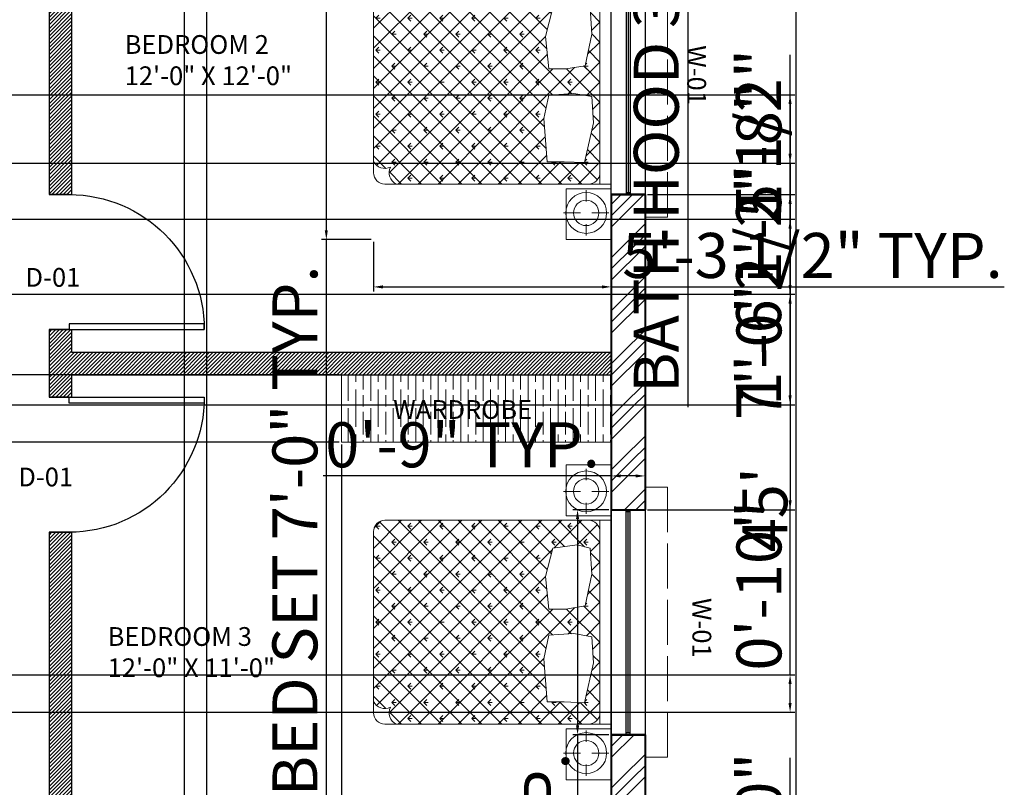
# Model space of a CAD drawing. Units: inches. Extents: x 2386 to 3029, y 792 to 1465.
# Tile 11 of 12: x 2724 to 2987, y 1044 to 1249. Entities that reach past the tile are written whole.
import ezdxf

# ---------------------------------------------------------------- set-up
doc = ezdxf.new("R2010")
doc.units = ezdxf.units.IN
doc.linetypes.add('ACAD_ISO02W100', pattern=[15, 12, -3])
for name, color, linetype, lineweight in [('A-AREA-IDEN', 4, 'Continuous', 25), ('A-DIMS', 1, 'Continuous', 18), ('A-DOOR', 2, 'Continuous', 25), ('A-FLOR-CASE', 6, 'Continuous', 18), ('A-FLOR-CASE-PATT', 9, 'Continuous', 13), ('A-FURN', 6, 'Continuous', 18), ('A-TEXT', 4, 'Continuous', 25), ('A-WALL-EXT', 7, 'Continuous', 40), ('A-WALL-INT', 9, 'Continuous', 30), ('A-WALL-PATT', 9, 'Continuous', 13), ('A-WINDOW', 4, 'Continuous', 25), ('A-WINDOW-OVHD', 4, 'ACAD_ISO02W100', 18)]:
    doc.layers.add(name, color=color, linetype=linetype, lineweight=lineweight)
doc.styles.get("Standard").update_dxf_attribs({"font": 'arial.ttf'})
doc.dimstyles.new('ISO-25', dxfattribs={"dimtxt": 12, "dimasz": 2.5, "dimexe": 1.25, "dimexo": 0.625, "dimtad": 1, "dimlunit": 4, "dimtxsty": 'Standard', "dimcen": 2.5, "dimadec": 0, "dimazin": 0, "dimtfac": 1, "dimtmove": 0, "dimatfit": 3, "dimfxl": 1, "dimarcsym": 0})

# ---------------------------------------------------------------- blocks, each defined once
blk = doc.blocks.new('*X5')
at = {"color": 0}
for p, q in [((0, 0), (0, 0)), ((-565.7, 0), (-565.7, 0)), ((-565.7, 0), (-565.7, 0)), ((-282.8, 0), (-282.8, 0)), ((-282.8, 0), (-282.8, 0)), ((282.8, 0), (282.8, 0)), ((565.7, 0), (565.7, 0)), ((-707.1, -141.4), (-733.6, -114.9)), ((-707.1, -141.4), (-707.1, -103.9)), ((-707.1, -141.4), (-680.6, -114.9)), ((-156.4, -126.5), (-167.9, -114.9)), ((-141.4, -141.4), (-142.5, -140.4)), ((-141.4, -141.4), (-141.4, -103.9)), ((-141.4, -141.4), (-114.9, -114.9)), ((119.7, -119.7), (114.9, -114.9)), ((699.4, -133.7), (680.6, -114.9)), ((707.1, -135.4), (707.1, -103.9)), ((710, -138.6), (733.6, -114.9)), ((-848.5, -282.8), (-875, -256.3)), ((-848.5, -282.8), (-848.5, -245.3)), ((-848.5, -282.8), (-822, -256.3)), ((0, -282.8), (-26.5, -256.3)), ((0, -282.8), (0, -245.3)), ((0, -282.8), (26.5, -256.3)), ((848.5, -282.8), (822, -256.3)), ((848.5, -282.8), (848.5, -245.3)), ((848.5, -282.8), (875, -256.3)), ((-707.1, -424.3), (-733.6, -397.7)), ((-707.1, -424.3), (-707.1, -386.8)), ((-707.1, -424.3), (-680.6, -397.7)), ((-115.7, -398.5), (-114.9, -397.7)), ((707.1, -424.3), (702.9, -420)), ((707.1, -424.3), (707.1, -386.8)), ((707.1, -424.3), (733.6, -397.7)), ((-848.5, -565.7), (-875, -539.2)), ((-848.5, -565.7), (-848.5, -528.2)), ((-848.5, -565.7), (-822, -539.2)), ((-565.7, -565.7), (-592.2, -539.2)), ((-565.7, -565.7), (-565.7, -528.2)), ((-565.7, -565.7), (-539.2, -539.2)), ((-282.8, -565.7), (-309.4, -539.2)), ((-282.8, -565.7), (-282.8, -528.2)), ((-282.8, -565.7), (-256.3, -539.2)), ((0, -565.7), (-26.5, -539.2)), ((0, -565.7), (0, -528.2)), ((0, -565.7), (26.5, -539.2)), ((282.8, -565.7), (256.3, -539.2)), ((282.8, -565.7), (282.8, -528.2)), ((282.8, -565.7), (309.4, -539.2)), ((565.7, -565.7), (539.2, -539.2)), ((565.7, -565.7), (565.7, -528.2)), ((565.7, -565.7), (592.2, -539.2)), ((848.5, -565.7), (822, -539.2)), ((848.5, -565.7), (848.5, -528.2)), ((848.5, -565.7), (875, -539.2)), ((-707.1, -707.1), (-733.6, -680.6)), ((-707.1, -707.1), (-707.1, -669.6)), ((-707.1, -707.1), (-680.6, -680.6)), ((-424.3, -707.1), (-450.8, -680.6)), ((-424.3, -707.1), (-424.3, -669.6)), ((-424.3, -707.1), (-397.7, -680.6)), ((-141.4, -707.1), (-167.9, -680.6)), ((-141.4, -707.1), (-141.4, -669.6)), ((-141.4, -707.1), (-114.9, -680.6)), ((141.4, -707.1), (114.9, -680.6)), ((141.4, -707.1), (141.4, -669.6)), ((141.4, -707.1), (167.9, -680.6)), ((424.3, -707.1), (397.7, -680.6)), ((424.3, -707.1), (424.3, -669.6)), ((424.3, -707.1), (450.8, -680.6)), ((707.1, -707.1), (680.6, -680.6)), ((707.1, -707.1), (707.1, -669.6)), ((707.1, -707.1), (733.6, -680.6)), ((-848.5, -848.5), (-875, -822)), ((-848.5, -848.5), (-848.5, -811)), ((-848.5, -848.5), (-822, -822)), ((-565.7, -848.5), (-592.2, -822)), ((-565.7, -848.5), (-565.7, -811)), ((-565.7, -848.5), (-539.2, -822)), ((-282.8, -848.5), (-309.4, -822)), ((-282.8, -848.5), (-282.8, -811)), ((-282.8, -848.5), (-256.3, -822)), ((0, -848.5), (-26.5, -822)), ((0, -848.5), (0, -811)), ((0, -848.5), (26.5, -822)), ((282.8, -848.5), (256.3, -822)), ((282.8, -848.5), (282.8, -811)), ((282.8, -848.5), (309.4, -822)), ((565.7, -848.5), (539.2, -822)), ((565.7, -848.5), (565.7, -811)), ((565.7, -848.5), (592.2, -822)), ((848.5, -848.5), (822, -822)), ((848.5, -848.5), (848.5, -811)), ((848.5, -848.5), (875, -822)), ((-707.1, -989.9), (-707.1, -952.4)), ((-424.3, -989.9), (-424.3, -952.4)), ((-141.4, -989.9), (-141.4, -952.4)), ((141.4, -989.9), (141.4, -952.4)), ((424.3, -989.9), (424.3, -952.4)), ((707.1, -989.9), (707.1, -952.4)), ((-707.1, -989.9), (-733.6, -963.4)), ((-707.1, -989.9), (-680.6, -963.4)), ((-424.3, -989.9), (-450.8, -963.4)), ((-424.3, -989.9), (-397.7, -963.4)), ((-141.4, -989.9), (-167.9, -963.4)), ((-141.4, -989.9), (-114.9, -963.4)), ((141.4, -989.9), (114.9, -963.4)), ((141.4, -989.9), (167.9, -963.4)), ((424.3, -989.9), (397.7, -963.4)), ((424.3, -989.9), (450.8, -963.4)), ((707.1, -989.9), (680.6, -963.4)), ((707.1, -989.9), (733.6, -963.4)), ((-848.5, -1131.4), (-875, -1104.9)), ((-848.5, -1131.4), (-848.5, -1093.9)), ((-848.5, -1131.4), (-822, -1104.9)), ((-565.7, -1131.4), (-592.2, -1104.9)), ((-565.7, -1131.4), (-565.7, -1093.9)), ((-565.7, -1131.4), (-539.2, -1104.9)), ((-282.8, -1131.4), (-309.4, -1104.9)), ((-282.8, -1131.4), (-282.8, -1093.9)), ((-282.8, -1131.4), (-256.3, -1104.9)), ((0, -1131.4), (-26.5, -1104.9)), ((0, -1131.4), (0, -1093.9)), ((0, -1131.4), (26.5, -1104.9)), ((282.8, -1131.4), (256.3, -1104.9)), ((282.8, -1131.4), (282.8, -1093.9)), ((282.8, -1131.4), (309.4, -1104.9)), ((565.7, -1131.4), (539.2, -1104.9)), ((565.7, -1131.4), (565.7, -1093.9)), ((565.7, -1131.4), (592.2, -1104.9)), ((848.5, -1131.4), (822, -1104.9)), ((848.5, -1131.4), (848.5, -1093.9)), ((848.5, -1131.4), (875, -1104.9)), ((-707.1, -1272.8), (-733.6, -1246.3)), ((-707.1, -1272.8), (-707.1, -1235.3)), ((-707.1, -1272.8), (-680.6, -1246.3)), ((-424.3, -1272.8), (-450.8, -1246.3)), ((-424.3, -1272.8), (-424.3, -1235.3)), ((-424.3, -1272.8), (-397.7, -1246.3)), ((-141.4, -1272.8), (-167.9, -1246.3)), ((-141.4, -1272.8), (-141.4, -1235.3)), ((-141.4, -1272.8), (-114.9, -1246.3)), ((141.4, -1272.8), (114.9, -1246.3)), ((141.4, -1272.8), (141.4, -1235.3)), ((141.4, -1272.8), (167.9, -1246.3)), ((424.3, -1272.8), (397.7, -1246.3)), ((424.3, -1272.8), (424.3, -1235.3)), ((424.3, -1272.8), (450.8, -1246.3)), ((707.1, -1272.8), (680.6, -1246.3)), ((707.1, -1272.8), (707.1, -1235.3)), ((707.1, -1272.8), (733.6, -1246.3)), ((-848.5, -1414.2), (-875, -1387.7)), ((-848.5, -1414.2), (-848.5, -1376.7)), ((-848.5, -1414.2), (-822, -1387.7)), ((-565.7, -1414.2), (-592.2, -1387.7)), ((-565.7, -1414.2), (-565.7, -1376.7)), ((-565.7, -1414.2), (-539.2, -1387.7)), ((-282.8, -1414.2), (-309.4, -1387.7)), ((-282.8, -1414.2), (-282.8, -1376.7)), ((-282.8, -1414.2), (-256.3, -1387.7)), ((0, -1414.2), (-26.5, -1387.7)), ((0, -1414.2), (0, -1376.7)), ((0, -1414.2), (26.5, -1387.7)), ((282.8, -1414.2), (256.3, -1387.7)), ((282.8, -1414.2), (282.8, -1376.7)), ((282.8, -1414.2), (309.4, -1387.7)), ((565.7, -1414.2), (539.2, -1387.7)), ((565.7, -1414.2), (565.7, -1376.7)), ((565.7, -1414.2), (592.2, -1387.7)), ((848.5, -1414.2), (822, -1387.7)), ((848.5, -1414.2), (848.5, -1376.7)), ((848.5, -1414.2), (875, -1387.7)), ((-707.1, -1555.6), (-733.6, -1529.1)), ((-707.1, -1555.6), (-707.1, -1518.1)), ((-707.1, -1555.6), (-680.6, -1529.1)), ((-424.3, -1555.6), (-450.8, -1529.1)), ((-424.3, -1555.6), (-424.3, -1518.1)), ((-424.3, -1555.6), (-397.7, -1529.1)), ((-141.4, -1555.6), (-167.9, -1529.1)), ((-141.4, -1555.6), (-141.4, -1518.1)), ((-141.4, -1555.6), (-114.9, -1529.1)), ((141.4, -1555.6), (114.9, -1529.1)), ((141.4, -1555.6), (141.4, -1518.1)), ((141.4, -1555.6), (167.9, -1529.1)), ((424.3, -1555.6), (397.7, -1529.1)), ((424.3, -1555.6), (424.3, -1518.1)), ((424.3, -1555.6), (450.8, -1529.1)), ((707.1, -1555.6), (680.6, -1529.1)), ((707.1, -1555.6), (707.1, -1518.1)), ((707.1, -1555.6), (733.6, -1529.1)), ((-848.5, -1697.1), (-875, -1670.5)), ((-848.5, -1697.1), (-848.5, -1659.6)), ((-848.5, -1697.1), (-822, -1670.5)), ((-565.7, -1697.1), (-592.2, -1670.5)), ((-565.7, -1697.1), (-565.7, -1659.6)), ((-565.7, -1697.1), (-539.2, -1670.5)), ((-282.8, -1697.1), (-309.4, -1670.5)), ((-282.8, -1697.1), (-282.8, -1659.6)), ((-282.8, -1697.1), (-256.3, -1670.5)), ((0, -1697.1), (-26.5, -1670.5)), ((0, -1697.1), (0, -1659.6)), ((0, -1697.1), (26.5, -1670.5)), ((282.8, -1697.1), (256.3, -1670.5)), ((282.8, -1697.1), (282.8, -1659.6)), ((282.8, -1697.1), (309.4, -1670.5)), ((565.7, -1697.1), (539.2, -1670.5)), ((565.7, -1697.1), (565.7, -1659.6)), ((565.7, -1697.1), (592.2, -1670.5)), ((848.5, -1697.1), (822, -1670.5)), ((848.5, -1697.1), (848.5, -1659.6)), ((848.5, -1697.1), (875, -1670.5)), ((-707.1, -1838.5), (-733.6, -1812)), ((-707.1, -1838.5), (-707.1, -1801)), ((-707.1, -1838.5), (-680.6, -1812)), ((-424.3, -1838.5), (-450.8, -1812)), ((-424.3, -1838.5), (-424.3, -1801)), ((-424.3, -1838.5), (-397.7, -1812)), ((-141.4, -1838.5), (-167.9, -1812)), ((-141.4, -1838.5), (-141.4, -1801)), ((-141.4, -1838.5), (-114.9, -1812)), ((141.4, -1838.5), (114.9, -1812)), ((141.4, -1838.5), (141.4, -1801)), ((141.4, -1838.5), (167.9, -1812)), ((424.3, -1838.5), (397.7, -1812)), ((424.3, -1838.5), (424.3, -1801)), ((424.3, -1838.5), (450.8, -1812)), ((707.1, -1838.5), (680.6, -1812)), ((707.1, -1838.5), (707.1, -1801)), ((707.1, -1838.5), (733.6, -1812)), ((-848.5, -1979.9), (-875, -1953.4)), ((-848.5, -1979.9), (-848.5, -1942.4)), ((-848.5, -1979.9), (-822, -1953.4)), ((-565.7, -1979.9), (-592.2, -1953.4)), ((-565.7, -1979.9), (-565.7, -1942.4)), ((-565.7, -1979.9), (-539.2, -1953.4)), ((-282.8, -1979.9), (-309.4, -1953.4)), ((-282.8, -1979.9), (-282.8, -1942.4)), ((-282.8, -1979.9), (-256.3, -1953.4)), ((0, -1979.9), (-26.5, -1953.4)), ((0, -1979.9), (0, -1942.4)), ((0, -1979.9), (26.5, -1953.4)), ((282.8, -1979.9), (256.3, -1953.4)), ((282.8, -1979.9), (282.8, -1942.4)), ((282.8, -1979.9), (309.4, -1953.4)), ((565.7, -1979.9), (539.2, -1953.4)), ((565.7, -1979.9), (565.7, -1942.4)), ((565.7, -1979.9), (592.2, -1953.4))]:
    blk.add_line(p, q, dxfattribs=at)
blk = doc.blocks.new('*X4')
at = {"color": 0}
for p, q in [((-900, -192.9), (-707.1, 0)), ((-623.2, -83.9), (-707.1, 0)), ((-613.7, -83.3), (-530.3, 0)), ((-456.8, -73.5), (-530.3, 0)), ((-425.1, -71.6), (-353.6, 0)), ((-245.3, -108.2), (-353.6, 0)), ((-278.3, -101.5), (-176.8, 0)), ((103, -279.8), (-176.8, 0)), ((-142.2, -142.2), (0, 0)), ((-116.9, -293.7), (176.8, 0)), ((119.7, -119.7), (0, 0)), ((241.2, -64.5), (176.8, 0)), ((292.3, -61.3), (353.6, 0)), ((425.9, -72.3), (353.6, 0)), ((452.1, -78.2), (530.3, 0)), ((653.8, -123.5), (530.3, 0)), ((596.5, -110.6), (707.1, 0)), ((900, -192.9), (707.1, 0)), ((-682.9, -201), (-862.2, -21.7)), ((708.5, -175.4), (862.2, -21.7)), ((-900, -369.7), (-666.9, -136.6)), ((-655.7, -405), (-900, -160.7)), ((702.9, -357.8), (900, -160.7)), ((-900, -1253.6), (101.2, -252.3)), ((900, -1253.6), (-128.3, -225.2)), ((900, -369.7), (708.4, -178.1)), ((-900, -546.4), (-667.8, -314.2)), ((735.1, -1972.5), (-900, -337.4)), ((-762.6, -2000), (900, -337.4)), ((-900, -1430.3), (111.9, -418.4)), ((-900, -723.2), (-605.3, -428.5)), ((801.1, -1861.8), (-641.4, -419.2)), ((900, -1430.3), (-115.7, -414.7)), ((900, -546.4), (702.9, -349.3)), ((-900, -900), (-464.7, -464.7)), ((-900, -1076.8), (-292.7, -469.5)), ((-900, -1607.1), (231.1, -476)), ((-900, -1783.9), (394.4, -489.4)), ((585.8, -2000), (-900, -514.2)), ((-887.6, -1948.2), (585.6, -475)), ((-585.8, -2000), (900, -514.2)), ((900, -1783.9), (-403.5, -480.4)), ((900, -1607.1), (-242.6, -464.5)), ((900, -1076.8), (317, -493.8)), ((900, -900), (482.8, -482.8)), ((900, -723.2), (647.2, -470.4)), ((409, -2000), (-900, -691)), ((-409, -2000), (900, -691)), ((232.2, -2000), (-900, -867.8)), ((-232.2, -2000), (900, -867.8)), ((55.5, -2000), (-900, -1044.5)), ((-55.5, -2000), (900, -1044.5)), ((-121.3, -2000), (-900, -1221.3)), ((121.3, -2000), (900, -1221.3)), ((-298.1, -2000), (-900, -1398.1)), ((298.1, -2000), (900, -1398.1)), ((-474.9, -2000), (-900, -1574.9)), ((474.9, -2000), (900, -1574.9)), ((-651.7, -2000), (-900, -1751.7)), ((790.3, -1861.4), (900, -1751.7)), ((651.7, -2000), (761.4, -1890.3)), ((-834.6, -1993.8), (-893.8, -1934.6))]:
    blk.add_line(p, q, dxfattribs=at)
blk = doc.blocks.new('A$C190D2546')
at = {"layer": 'A-FURN'}
for p, q in [((540.9, 2100), (2340.9, 2100)), ((540.9, 1880.7), (540.9, 2100)), ((2340.9, 1880.7), (2340.9, 2100)), ((285.2, 1928.3), (285.2, 2078.3)), ((2596, 1929), (2596, 2079)), ((2340.9, 2000), (540.9, 2000)), ((185.2, 1878.3), (85.2, 1878.3)), ((285.2, 1828.3), (285.2, 1678.3)), ((385.2, 1878.3), (485.2, 1878.3)), ((2496, 1879), (2396, 1879)), ((2596, 1829), (2596, 1679)), ((2696, 1879), (2796, 1879))]:
    blk.add_line(p, q, dxfattribs=at)
for points in [[(500, 2100.7), (500, 1700.7), (50, 1700.7), (50, 2100.7)], [(2381.8, 2100.7), (2381.8, 1700.7), (2831.8, 1700.7), (2831.8, 2100.7)], [(786.7, 1584.1), (758, 1799.3), (786.7, 1914.1), (1016.5, 1928.5), (1296.5, 1871.1), (1325.2, 1698.9), (1325.2, 1548.2), (1038, 1519.5)], [(1555, 1548.2), (1540.6, 1770.6), (1569.4, 1928.5), (1799.1, 1942.8), (2151, 1863.9), (2143.8, 1684.5), (2143.8, 1533.8), (1763.2, 1505.1)]]:
    blk.add_lwpolyline(points, close=True, dxfattribs=at)
blk.add_lwpolyline([(640.9, 2000), (2240.9, 2000, -0.414214), (2340.9, 1900), (2340.9, 100, -0.414214), (2240.9, 0), (640.9, 0, -0.414214), (540.9, 100), (540.9, 1900, -0.414214)], format="xyb", close=True, dxfattribs=at)
for centre, radius in [((285.2, 1878.3), 180.3), ((2596, 1879), 180.3), ((285.2, 1878.3), 111.8), ((2596, 1879), 111.8)]:
    blk.add_circle(centre, radius, dxfattribs=at)
for centre, start, end in [((2240.9, 250), 243.43495, 333.43495), ((2090.9, 100), 296.56505, 26.56505)]:
    blk.add_arc(centre, 111.8, start, end, dxfattribs=at)
for name in ['*X4', '*X5']:
    blk.add_blockref(name, (1440.9, 2000), dxfattribs=at)
blk = doc.blocks.new('*U2')
for p, q in [((0, 0), (0, -6)), ((40, 0), (40, -6))]:
    blk.add_line(p, q)
blk.add_lwpolyline([(0, 0), (0, 40), (1.75, 40), (1.75, 0)], close=True)
blk.add_arc((0, 0), 40, 0, 90)
blk = doc.blocks.new('*U3')
for p, q in [((0, 0), (0, -6)), ((-40, 0), (-40, -6))]:
    blk.add_line(p, q)
blk.add_lwpolyline([(0, 0), (0, 40), (-1.75, 40), (-1.75, 0)], close=True)
blk.add_arc((0, 0), 40, 90, 180)
blk = doc.blocks.new('*D22')
at = {"layer": 'A-DIMS', "color": 0, "lineweight": -2, "transparency": 16777216}
for p, q in [((2891.82, 1387.95), (2932.69, 1387.95)), ((2931.44, 1385.45), (2931.44, 850.45)), ((2891.82, 847.95), (2932.69, 847.95))]:
    blk.add_line(p, q, dxfattribs=at)
at = {"layer": 'A-DIMS', "color": 0, "transparency": 16777216}
for points in [[(2931.02, 1385.45), (2931.85, 1385.45), (2931.44, 1387.95)], [(2931.02, 850.45), (2931.85, 850.45), (2931.44, 847.95)]]:
    blk.add_solid(points, dxfattribs=at)
at = {"layer": 'Defpoints', "color": 0, "transparency": 16777216}
for p in [(2891.19, 1387.95), (2891.19, 847.95), (2931.44, 847.95)]:
    blk.add_point(p, dxfattribs=at)
at = {"layer": 'A-DIMS', "color": 0, "transparency": 16777216, "insert": (2924.71, 1117.95), "char_height": 12, "attachment_point": 5, "rotation": 90}
blk.add_mtext("45'", dxfattribs=at)
blk = doc.blocks.new('WINDOW-60IN')
for p, q in [((0, 0), (0, 60)), ((0, 60), (9, 60)), ((4, 60), (4, 0)), ((4, 59.5), (5, 59.5)), ((4.5, 59.5), (4.5, 0.5)), ((5, 60), (5, 0)), ((9, 60), (9, 0)), ((0, 0), (9, 0)), ((5, 0.5), (4, 0.5))]:
    blk.add_line(p, q)
blk = doc.blocks.new('WINDOW-HOOD-60IN')
for p, q in [((0, 72), (6, 72)), ((6, 72), (6, 0)), ((0, 0), (6, 0))]:
    blk.add_line(p, q)
blk = doc.blocks.new('*D34')
at = {"layer": 'A-DIMS', "color": 0, "lineweight": -2, "transparency": 16777216}
for p, q in [((2818.13, 1273.95), (2804.91, 1273.95)), ((2806.16, 1271.45), (2806.16, 1192.45)), ((2818.13, 1189.95), (2804.91, 1189.95)), ((2806.16, 1189.95), (2806.16, 1037.2))]:
    blk.add_line(p, q, dxfattribs=at)
at = {"layer": 'A-DIMS', "color": 0, "transparency": 16777216}
for points in [[(2805.74, 1271.45), (2806.57, 1271.45), (2806.16, 1273.95)], [(2805.74, 1192.45), (2806.57, 1192.45), (2806.16, 1189.95)]]:
    blk.add_solid(points, dxfattribs=at)
at = {"layer": 'Defpoints', "color": 0, "transparency": 16777216}
for p in [(2818.76, 1273.95), (2806.16, 1189.95), (2818.76, 1189.95)]:
    blk.add_point(p, dxfattribs=at)
at = {"layer": 'A-DIMS', "color": 0, "transparency": 16777216, "insert": (2799.33, 1112.32), "char_height": 12, "attachment_point": 5, "rotation": 90}
blk.add_mtext('BED SET 7\'-0" TYP.', dxfattribs=at)
blk = doc.blocks.new('*D35')
at = {"layer": 'A-DIMS', "color": 0, "lineweight": -2, "transparency": 16777216}
for p, q in [((2818.76, 1189.32), (2818.76, 1176.1)), ((2882.19, 1189.32), (2882.19, 1176.1)), ((2821.26, 1177.35), (2879.69, 1177.35)), ((2882.19, 1177.35), (2987.05, 1177.35))]:
    blk.add_line(p, q, dxfattribs=at)
at = {"layer": 'A-DIMS', "color": 0, "transparency": 16777216}
for points in [[(2821.26, 1177.76), (2821.26, 1176.93), (2818.76, 1177.35)], [(2879.69, 1177.76), (2879.69, 1176.93), (2882.19, 1177.35)]]:
    blk.add_solid(points, dxfattribs=at)
at = {"layer": 'Defpoints', "color": 0, "transparency": 16777216}
for p in [(2818.76, 1189.95), (2882.19, 1189.95), (2882.19, 1177.35)]:
    blk.add_point(p, dxfattribs=at)
at = {"layer": 'A-DIMS', "color": 0, "transparency": 16777216, "insert": (2935.87, 1184.18), "char_height": 12, "attachment_point": 5}
blk.add_mtext('5\'-3 1/2" TYP.', dxfattribs=at)
blk = doc.blocks.new('*D36')
at = {"layer": 'A-DIMS', "color": 0, "lineweight": -2, "transparency": 16777216}
for p, q in [((2881.57, 1117.95), (2871.94, 1117.95)), ((2873.19, 1115.45), (2873.19, 1060.45)), ((2881.57, 1057.95), (2871.94, 1057.95)), ((2873.19, 1057.95), (2873.19, 935.85))]:
    blk.add_line(p, q, dxfattribs=at)
at = {"layer": 'A-DIMS', "color": 0, "transparency": 16777216}
for points in [[(2872.77, 1115.45), (2873.61, 1115.45), (2873.19, 1117.95)], [(2872.77, 1060.45), (2873.61, 1060.45), (2873.19, 1057.95)]]:
    blk.add_solid(points, dxfattribs=at)
at = {"layer": 'Defpoints', "color": 0, "transparency": 16777216}
for p in [(2882.19, 1117.95), (2873.19, 1057.95), (2882.19, 1057.95)]:
    blk.add_point(p, dxfattribs=at)
at = {"layer": 'A-DIMS', "color": 0, "transparency": 16777216, "insert": (2866.44, 995.65), "char_height": 12, "attachment_point": 5, "rotation": 90}
blk.add_mtext('W-01 5\'-0" TYP.', dxfattribs=at)
blk = doc.blocks.new('*D37')
at = {"layer": 'A-DIMS', "color": 0, "lineweight": -2, "transparency": 16777216}
for p, q in [((2882.19, 1118.57), (2882.19, 1128.2)), ((2891.19, 1118.57), (2891.19, 1128.2)), ((2882.19, 1126.95), (2805.29, 1126.95)), ((2888.69, 1126.95), (2884.69, 1126.95))]:
    blk.add_line(p, q, dxfattribs=at)
at = {"layer": 'A-DIMS', "color": 0, "transparency": 16777216}
for points in [[(2884.69, 1127.36), (2884.69, 1126.53), (2882.19, 1126.95)], [(2888.69, 1127.36), (2888.69, 1126.53), (2891.19, 1126.95)]]:
    blk.add_solid(points, dxfattribs=at)
at = {"layer": 'Defpoints', "color": 0, "transparency": 16777216}
for p in [(2882.19, 1126.95), (2882.19, 1117.95), (2891.19, 1117.95)]:
    blk.add_point(p, dxfattribs=at)
at = {"layer": 'A-DIMS', "color": 0, "transparency": 16777216, "insert": (2842.49, 1133.7), "char_height": 12, "attachment_point": 5}
blk.add_mtext('0\'-9" TYP.', dxfattribs=at)
blk = doc.blocks.new('*D50')
at = {"layer": 'A-DIMS', "color": 0, "lineweight": -2, "transparency": 16777216}
for p, q in [((2897.82, 1361.95), (2903.84, 1361.95)), ((2902.59, 1359.45), (2902.59, 1328.45)), ((2897.82, 1325.95), (2903.84, 1325.95)), ((2902.59, 1325.95), (2902.59, 1145.27))]:
    blk.add_line(p, q, dxfattribs=at)
at = {"layer": 'A-DIMS', "color": 0, "transparency": 16777216}
for points in [[(2902.17, 1359.45), (2903.01, 1359.45), (2902.59, 1361.95)], [(2902.17, 1328.45), (2903.01, 1328.45), (2902.59, 1325.95)]]:
    blk.add_solid(points, dxfattribs=at)
at = {"layer": 'Defpoints', "color": 0, "transparency": 16777216}
for p in [(2897.19, 1361.95), (2897.19, 1325.95), (2902.59, 1325.95)]:
    blk.add_point(p, dxfattribs=at)
at = {"layer": 'A-DIMS', "color": 0, "transparency": 16777216, "insert": (2895.75, 1234.36), "char_height": 12, "attachment_point": 5, "rotation": 90}
blk.add_mtext('BATH HOOD 3\'-0" TYP.', dxfattribs=at)
blk = doc.blocks.new('*D59')
at = {"layer": 'A-DIMS', "color": 0, "lineweight": -2, "transparency": 16777216}
for p, q in [((2768.19, 1308.32), (2768.19, 808)), ((2774.19, 1308.32), (2774.19, 808)), ((2765.69, 809.25), (2763.19, 809.25)), ((2768.19, 809.25), (2774.19, 809.25)), ((2776.69, 809.25), (2812.34, 809.25))]:
    blk.add_line(p, q, dxfattribs=at)
at = {"layer": 'A-DIMS', "color": 0, "transparency": 16777216}
for points in [[(2765.69, 809.66), (2765.69, 808.83), (2768.19, 809.25)], [(2776.69, 809.66), (2776.69, 808.83), (2774.19, 809.25)]]:
    blk.add_solid(points, dxfattribs=at)
at = {"layer": 'Defpoints', "color": 0, "transparency": 16777216}
for p in [(2768.19, 1308.95), (2774.19, 1308.95), (2774.19, 809.25)]:
    blk.add_point(p, dxfattribs=at)
at = {"layer": 'A-DIMS', "color": 0, "transparency": 16777216, "insert": (2795.76, 816), "char_height": 12, "attachment_point": 5}
blk.add_mtext('0\'-6"', dxfattribs=at)
blk = doc.blocks.new('*D69')
at = {"layer": 'A-DIMS', "color": 0, "lineweight": -2, "transparency": 16777216}
for p, q in [((2891.82, 1201.95), (2931.14, 1201.95)), ((2929.89, 1199.45), (2929.89, 1120.45)), ((2891.82, 1117.95), (2931.14, 1117.95))]:
    blk.add_line(p, q, dxfattribs=at)
at = {"layer": 'A-DIMS', "color": 0, "transparency": 16777216}
for points in [[(2929.47, 1199.45), (2930.31, 1199.45), (2929.89, 1201.95)], [(2929.47, 1120.45), (2930.31, 1120.45), (2929.89, 1117.95)]]:
    blk.add_solid(points, dxfattribs=at)
at = {"layer": 'Defpoints', "color": 0, "transparency": 16777216}
for p in [(2891.19, 1201.95), (2891.19, 1117.95), (2929.89, 1117.95)]:
    blk.add_point(p, dxfattribs=at)
at = {"layer": 'A-DIMS', "color": 0, "transparency": 16777216, "insert": (2923.14, 1159.95), "char_height": 12, "attachment_point": 5, "rotation": 90}
blk.add_mtext('7\'-0"', dxfattribs=at)
blk = doc.blocks.new('*D75')
at = {"layer": 'A-DIMS', "color": 0, "lineweight": -2, "transparency": 16777216}
for p, q in [((2929.89, 1195.39), (2929.89, 1229.91)), ((2498.82, 1195.39), (2931.14, 1195.39)), ((2929.89, 1177.89), (2929.89, 1192.89)), ((2498.82, 1175.39), (2931.14, 1175.39))]:
    blk.add_line(p, q, dxfattribs=at)
at = {"layer": 'A-DIMS', "color": 0, "transparency": 16777216}
for points in [[(2929.47, 1192.89), (2930.31, 1192.89), (2929.89, 1195.39)], [(2929.47, 1177.89), (2930.31, 1177.89), (2929.89, 1175.39)]]:
    blk.add_solid(points, dxfattribs=at)
at = {"layer": 'Defpoints', "color": 0, "transparency": 16777216}
for p in [(2498.19, 1195.39), (2929.89, 1195.39), (2498.19, 1175.39)]:
    blk.add_point(p, dxfattribs=at)
at = {"layer": 'A-DIMS', "color": 0, "transparency": 16777216, "insert": (2923.14, 1213.9), "char_height": 12, "attachment_point": 5, "rotation": 90}
blk.add_mtext('1\'-8"', dxfattribs=at)
blk = doc.blocks.new('*D79')
at = {"layer": 'A-DIMS', "color": 0, "lineweight": -2, "transparency": 16777216}
for p, q in [((2929.89, 1073.95), (2929.89, 1118.92)), ((2516.82, 1073.95), (2931.14, 1073.95)), ((2929.89, 1066.45), (2929.89, 1071.45)), ((2516.82, 1063.95), (2931.14, 1063.95))]:
    blk.add_line(p, q, dxfattribs=at)
at = {"layer": 'A-DIMS', "color": 0, "transparency": 16777216}
for points in [[(2929.47, 1071.45), (2930.31, 1071.45), (2929.89, 1073.95)], [(2929.47, 1066.45), (2930.31, 1066.45), (2929.89, 1063.95)]]:
    blk.add_solid(points, dxfattribs=at)
at = {"layer": 'Defpoints', "color": 0, "transparency": 16777216}
for p in [(2516.19, 1073.95), (2929.89, 1073.95), (2516.19, 1063.95)]:
    blk.add_point(p, dxfattribs=at)
at = {"layer": 'A-DIMS', "color": 0, "transparency": 16777216, "insert": (2923.14, 1097.68), "char_height": 12, "attachment_point": 5, "rotation": 90}
blk.add_mtext('0\'-10"', dxfattribs=at)
blk = doc.blocks.new('*D80')
at = {"layer": 'A-DIMS', "color": 0, "lineweight": -2, "transparency": 16777216}
for p, q in [((2810.19, 1135.32), (2810.19, 808)), ((2882.19, 1135.32), (2882.19, 808)), ((2812.69, 809.25), (2879.69, 809.25))]:
    blk.add_line(p, q, dxfattribs=at)
at = {"layer": 'A-DIMS', "color": 0, "transparency": 16777216}
for points in [[(2812.69, 809.66), (2812.69, 808.83), (2810.19, 809.25)], [(2879.69, 809.66), (2879.69, 808.83), (2882.19, 809.25)]]:
    blk.add_solid(points, dxfattribs=at)
at = {"layer": 'Defpoints', "color": 0, "transparency": 16777216}
for p in [(2810.19, 1135.95), (2882.19, 1135.95), (2882.19, 809.25)]:
    blk.add_point(p, dxfattribs=at)
at = {"layer": 'A-DIMS', "color": 0, "transparency": 16777216, "insert": (2846.19, 816), "char_height": 12, "attachment_point": 5}
blk.add_mtext('6\'-0"', dxfattribs=at)
blk = doc.blocks.new('*D81')
at = {"layer": 'A-DIMS', "color": 0, "lineweight": -2, "transparency": 16777216}
for p, q in [((2432.49, 1153.95), (2432.49, 1188.47)), ((2809.57, 1153.95), (2431.24, 1153.95)), ((2432.49, 1138.45), (2432.49, 1151.45)), ((2809.57, 1135.95), (2431.24, 1135.95))]:
    blk.add_line(p, q, dxfattribs=at)
at = {"layer": 'A-DIMS', "color": 0, "transparency": 16777216}
for points in [[(2432.07, 1151.45), (2432.91, 1151.45), (2432.49, 1153.95)], [(2432.07, 1138.45), (2432.91, 1138.45), (2432.49, 1135.95)]]:
    blk.add_solid(points, dxfattribs=at)
at = {"layer": 'Defpoints', "color": 0, "transparency": 16777216}
for p in [(2432.49, 1153.95), (2810.19, 1153.95), (2810.19, 1135.95)]:
    blk.add_point(p, dxfattribs=at)
at = {"layer": 'A-DIMS', "color": 0, "transparency": 16777216, "insert": (2425.74, 1172.46), "char_height": 12, "attachment_point": 5, "rotation": 90}
blk.add_mtext('1\'-6"', dxfattribs=at)
blk = doc.blocks.new('*D86')
at = {"layer": 'A-DIMS', "color": 0, "lineweight": -2, "transparency": 16777216}
for p, q in [((2929.89, 1015.95), (2929.89, 1051.8)), ((2882.82, 1015.95), (2931.14, 1015.95)), ((2929.89, 994.45), (2929.89, 1013.45)), ((2858.82, 991.95), (2931.14, 991.95))]:
    blk.add_line(p, q, dxfattribs=at)
at = {"layer": 'A-DIMS', "color": 0, "transparency": 16777216}
for points in [[(2929.47, 1013.45), (2930.31, 1013.45), (2929.89, 1015.95)], [(2929.47, 994.45), (2930.31, 994.45), (2929.89, 991.95)]]:
    blk.add_solid(points, dxfattribs=at)
at = {"layer": 'Defpoints', "color": 0, "transparency": 16777216}
for p in [(2882.19, 1015.95), (2929.89, 1015.95), (2858.19, 991.95)]:
    blk.add_point(p, dxfattribs=at)
at = {"layer": 'A-DIMS', "color": 0, "transparency": 16777216, "insert": (2923.14, 1035.12), "char_height": 12, "attachment_point": 5, "rotation": 90}
blk.add_mtext('2\'-0"', dxfattribs=at)
blk = doc.blocks.new('*D100')
at = {"layer": 'A-DIMS', "color": 0, "lineweight": -2, "transparency": 16777216}
for p, q in [((2562.86, 1228.59), (2931.14, 1228.59)), ((2929.89, 1226.09), (2929.89, 1212.84)), ((2563.05, 1210.34), (2931.14, 1210.34)), ((2929.89, 1210.34), (2929.89, 1147.86))]:
    blk.add_line(p, q, dxfattribs=at)
at = {"layer": 'A-DIMS', "color": 0, "transparency": 16777216}
for points in [[(2929.47, 1226.09), (2930.31, 1226.09), (2929.89, 1228.59)], [(2929.47, 1212.84), (2930.31, 1212.84), (2929.89, 1210.34)]]:
    blk.add_solid(points, dxfattribs=at)
at = {"layer": 'Defpoints', "color": 0, "transparency": 16777216}
for p in [(2562.24, 1228.59), (2562.43, 1210.34), (2929.89, 1210.34)]:
    blk.add_point(p, dxfattribs=at)
at = {"layer": 'A-DIMS', "color": 0, "transparency": 16777216, "insert": (2923.06, 1177.85), "char_height": 12, "attachment_point": 5, "rotation": 90}
blk.add_mtext('1\'-6 1/2"', dxfattribs=at)
blk = doc.blocks.new('*D101')
at = {"layer": 'A-DIMS', "color": 0, "lineweight": -2, "transparency": 16777216}
for p, q in [((2929.89, 1175.39), (2929.89, 1239.21)), ((2480.82, 1175.39), (2931.14, 1175.39)), ((2929.89, 1148.45), (2929.89, 1172.89)), ((2480.82, 1145.95), (2931.14, 1145.95))]:
    blk.add_line(p, q, dxfattribs=at)
at = {"layer": 'A-DIMS', "color": 0, "transparency": 16777216}
for points in [[(2929.47, 1172.89), (2930.31, 1172.89), (2929.89, 1175.39)], [(2929.47, 1148.45), (2930.31, 1148.45), (2929.89, 1145.95)]]:
    blk.add_solid(points, dxfattribs=at)
at = {"layer": 'Defpoints', "color": 0, "transparency": 16777216}
for p in [(2480.19, 1175.39), (2929.89, 1175.39), (2480.19, 1145.95)]:
    blk.add_point(p, dxfattribs=at)
at = {"layer": 'A-DIMS', "color": 0, "transparency": 16777216, "insert": (2923.06, 1208.55), "char_height": 12, "attachment_point": 5, "rotation": 90}
blk.add_mtext('2\'-5 1/2"', dxfattribs=at)

msp = doc.modelspace()

# ---------------------------------------------------------------- hatches: boundary and pattern name
at = {"layer": 'A-FLOR-CASE-PATT'}
h = msp.add_hatch(dxfattribs=at)
h.set_pattern_fill('GOST_WOOD', color=256)
h.paths.add_polyline_path([(2810.19, 1135.948), (2882.19, 1135.948), (2882.19, 1153.948), (2810.19, 1153.948)])
h.paths.add_polyline_path([(2822.689, 1139.339), (2866.325, 1139.339), (2866.325, 1149.643), (2822.689, 1149.643)], flags=24)
at = {"layer": 'A-WALL-PATT'}
h = msp.add_hatch(dxfattribs=at)
h.set_pattern_fill('GOST_GROUND', color=256)
h.paths.add_polyline_path([(2480.19, 1276.948), (2471.19, 1276.948), (2471.19, 1211.948), (2480.19, 1211.948)])
h.paths.add_polyline_path([(2480.19, 1378.948), (2510.19, 1378.948), (2510.19, 1378.969), (2523.779, 1378.969), (2580.602, 1378.959), (2580.602, 1378.969), (2594.19, 1378.969), (2642.19, 1378.948), (2642.19, 1387.948), (2471.19, 1387.948), (2471.19, 1336.948), (2480.19, 1336.948)])
h.paths.add_polyline_path([(2891.19, 1387.948), (2666.19, 1387.948), (2666.19, 1378.948), (2882.19, 1378.948), (2882.19, 1355.948), (2891.19, 1355.948)])
h.paths.add_polyline_path([(2891.19, 1331.948), (2882.19, 1331.948), (2882.19, 1331.449), (2882.19, 1261.948), (2891.19, 1261.948)])
h.paths.add_polyline_path([(2891.19, 1201.948), (2882.19, 1201.948), (2882.19, 1189.948), (2882.19, 1159.948), (2882.19, 1117.948), (2891.19, 1117.948)])
h.paths.add_polyline_path([(2891.19, 1057.948), (2882.19, 1057.948), (2882.19, 856.948), (2882.19, 847.948), (2891.19, 847.948)])
h.paths.add_polyline_path([(2594.19, 856.948), (2558.19, 856.948), (2558.19, 847.948), (2594.19, 847.948)])
h.paths.add_polyline_path([(2510.19, 856.948), (2480.19, 856.948), (2480.19, 905.448), (2471.19, 905.448), (2471.19, 847.948), (2510.19, 847.948)])
h.paths.add_polyline_path([(2480.19, 1007.948), (2471.19, 1007.948), (2471.19, 953.448), (2480.19, 953.448)])
h.paths.add_polyline_path([(2480.19, 1103.948), (2471.19, 1103.948), (2471.19, 1043.948), (2480.19, 1043.948)])
h = msp.add_hatch(dxfattribs=at)
h.set_pattern_fill('JIS_WOOD', color=256)
h.paths.add_polyline_path([(2624.19, 1229.948), (2624.19, 1145.948), (2618.19, 1145.948), (2618.19, 1140.548), (2618.19, 1139.948), (2630.19, 1139.948), (2630.19, 1240.948), (2624.19, 1240.948), (2624.19, 1234.948), (2480.19, 1234.948), (2480.19, 1229.948)])
h.paths.add_polyline_path([(2582.19, 1139.948), (2582.19, 1145.948), (2480.19, 1145.948), (2480.19, 1139.948)], flags=17)
h.paths.add_polyline_path([(2480.19, 1007.948), (2480.19, 1001.948), (2546.19, 1001.948), (2546.19, 1007.348), (2546.19, 1007.948)])
h.paths.add_polyline_path([(2594.19, 1007.948), (2582.19, 1007.948), (2582.19, 1001.948), (2588.19, 1001.948), (2588.19, 856.948), (2594.19, 856.948), (2594.19, 914.948), (2606.19, 914.948), (2606.19, 920.948), (2594.19, 920.948)])
h.paths.add_polyline_path([(2738.19, 1015.948), (2882.19, 1015.948), (2882.19, 1021.948), (2738.19, 1021.948), (2738.19, 1111.948), (2732.19, 1111.948), (2732.19, 920.948), (2720.19, 920.948), (2720.19, 914.948), (2732.19, 914.948), (2732.19, 856.948), (2738.19, 856.948)])
h.paths.add_polyline_path([(2660.19, 914.948), (2660.19, 920.948), (2648.19, 920.948), (2648.19, 914.948)])
h.paths.add_polyline_path([(2738.19, 1159.948), (2738.19, 1165.948), (2737.59, 1165.948), (2732.19, 1165.948), (2732.19, 1147.948), (2737.59, 1147.948), (2738.19, 1147.948), (2738.19, 1153.948), (2882.19, 1153.948), (2882.19, 1159.948)])
h.paths.add_polyline_path([(2732.19, 1201.948), (2738.19, 1201.948), (2738.19, 1303.948), (2774.19, 1303.948), (2774.19, 1308.948), (2768.19, 1308.948), (2768.19, 1378.948), (2762.19, 1378.948), (2762.19, 1308.948), (2726.19, 1308.948), (2726.19, 1303.948), (2732.19, 1303.948)])
h.paths.add_polyline_path([(2696.19, 1303.948), (2696.19, 1308.948), (2630.19, 1308.948), (2630.19, 1378.948), (2624.19, 1378.948), (2624.19, 1276.948), (2630.19, 1276.948), (2630.19, 1303.948)])

# ---------------------------------------------------------------- linework, layer by layer
at = {"layer": 'A-FLOR-CASE'}
msp.add_lwpolyline([(2810.19, 1153.948), (2810.19, 1135.948), (2882.19, 1135.948)], dxfattribs=at)
at = {"layer": 'A-WALL-EXT'}
for p, q in [((2882.19, 1201.948), (2882.19, 1159.948)), ((2882.19, 1201.948), (2891.19, 1201.948)), ((2891.19, 1201.948), (2882.19, 1201.948)), ((2891.19, 1201.948), (2891.19, 1117.948)), ((2882.19, 1159.948), (2882.19, 1117.948)), ((2882.19, 1117.948), (2891.19, 1117.948)), ((2882.19, 1117.948), (2891.19, 1117.948)), ((2882.19, 1057.948), (2882.19, 856.948)), ((2882.19, 1057.948), (2891.19, 1057.948)), ((2891.19, 1057.948), (2882.19, 1057.948)), ((2891.19, 1057.948), (2891.19, 847.948))]:
    msp.add_line(p, q, dxfattribs=at)
at = {"layer": 'A-WALL-INT'}
for p, q in [((2732.19, 1303.948), (2732.19, 1201.948)), ((2738.19, 1303.948), (2738.19, 1201.948)), ((2732.19, 1201.948), (2738.19, 1201.948)), ((2732.19, 1165.948), (2738.19, 1165.948)), ((2732.19, 1165.948), (2732.19, 1147.948)), ((2738.19, 1165.948), (2738.19, 1159.948)), ((2738.19, 1159.948), (2882.19, 1159.948)), ((2738.19, 1153.948), (2882.19, 1153.948)), ((2738.19, 1153.948), (2738.19, 1147.948)), ((2732.19, 1147.948), (2738.19, 1147.948)), ((2732.19, 1111.948), (2738.19, 1111.948)), ((2732.19, 1111.948), (2732.19, 920.948)), ((2738.19, 1111.948), (2738.19, 1021.948))]:
    msp.add_line(p, q, dxfattribs=at)

# ---------------------------------------------------------------- block references
at = {"layer": 'A-DOOR', "xscale": -0.9, "yscale": 0.9, "zscale": 0.9, "rotation": 270}
for name, p in [('*U2', (2737.59, 1165.948)), ('*U3', (2737.59, 1147.948))]:
    msp.add_blockref(name, p, dxfattribs=at)
at = {"layer": 'A-FURN', "xscale": 0.0301964232523521, "yscale": 0.0301964232523521, "zscale": 0.0301964232523521, "rotation": 270}
for p in [(2818.757, 1275.458), (2818.757, 1131.458)]:
    msp.add_blockref('A$C190D2546', p, dxfattribs=at)
at = {"layer": 'A-WINDOW'}
msp.add_blockref('WINDOW-60IN', (2882.19, 1201.948), dxfattribs=at)
at = {"layer": 'A-WINDOW', "rotation": 180}
msp.add_blockref('WINDOW-60IN', (2891.19, 1117.948), dxfattribs=at)
at = {"layer": 'A-WINDOW-OVHD'}
for p in [(2891.19, 1195.948), (2891.19, 1051.948)]:
    msp.add_blockref('WINDOW-HOOD-60IN', p, dxfattribs=at)

# ---------------------------------------------------------------- texts
at = {"layer": 'A-AREA-IDEN', "char_height": 5, "attachment_point": 1}
for s, insert in [('BEDROOM 2\\P12\'-0" X 12\'-0"', (2752.348, 1244.47)), ('WARDROBE', (2824.024, 1147.158)), ('BEDROOM 3\\P12\'-0" X 11\'-0"', (2747.807, 1086.643))]:
    msp.add_mtext_dynamic_manual_height_columns(s, width=52.37406, gutter_width=12.5, heights=[0], dxfattribs=dict(at, insert=insert))
at = {"layer": 'A-TEXT', "char_height": 5, "attachment_point": 1, "rotation": 270}
for insert in [(2907.46, 1241.783), (2908.853, 1094.42)]:
    msp.add_mtext_dynamic_manual_height_columns('W-01', width=38.22215, gutter_width=12.5, heights=[0], dxfattribs=dict(at, insert=insert))
at = {"layer": 'A-TEXT', "char_height": 5, "attachment_point": 1}
for insert in [(2725.89, 1182.384), (2723.971, 1129.167)]:
    msp.add_mtext_dynamic_manual_height_columns('D-01', width=38.22215, gutter_width=12.5, heights=[0], dxfattribs=dict(at, insert=insert))

# ---------------------------------------------------------------- dimensions: what is measured, and where the dimension line sits
at = {"layer": 'A-DIMS'}
for base, p1, p2, override, picture, middle in [((2931.437, 847.948), (2891.19, 1387.948), (2891.19, 847.948), {"dimclrd": 0, "dimclre": 0, "dimclrt": 0}, '*D22', (2924.709, 1117.948)), ((2929.89, 1175.392), (2480.19, 1145.948), (2480.19, 1175.392), {"dimdec": 1, "dimlfac": 1, "dimrnd": 0, "dimzin": 1, "dimdsep": 46, "dimlunit": 4, "dimfrac": 2}, '*D101', (2923.06, 1208.55)), ((2929.89, 1195.392), (2498.19, 1175.392), (2498.19, 1195.392), {"dimdec": 1, "dimlfac": 1, "dimrnd": 0, "dimzin": 1, "dimdsep": 46, "dimlunit": 4, "dimfrac": 2}, '*D75', (2923.138, 1213.902)), ((2929.89, 1210.342), (2562.236, 1228.595), (2562.425, 1210.342), {"dimdec": 1, "dimlfac": 1, "dimrnd": 0, "dimzin": 1, "dimdsep": 46, "dimlunit": 4, "dimfrac": 2}, '*D100', (2923.06, 1177.852)), ((2929.89, 1117.948), (2891.19, 1201.948), (2891.19, 1117.948), {"dimdec": 1, "dimlfac": 1, "dimrnd": 0, "dimzin": 1, "dimdsep": 46, "dimlunit": 4, "dimfrac": 2}, '*D69', (2923.138, 1159.948)), ((2432.49, 1153.948), (2810.19, 1135.948), (2810.19, 1153.948), {"dimdec": 1, "dimlfac": 1, "dimrnd": 0, "dimzin": 1, "dimdsep": 46, "dimlunit": 4, "dimfrac": 2}, '*D81', (2425.738, 1172.458)), ((2929.89, 1073.948), (2516.19, 1063.948), (2516.19, 1073.948), {"dimdec": 1, "dimlfac": 1, "dimrnd": 0, "dimzin": 1, "dimdsep": 46, "dimlunit": 4, "dimfrac": 2}, '*D79', (2923.138, 1097.684)), ((2929.89, 1015.948), (2858.19, 991.948), (2882.19, 1015.948), {"dimdec": 1, "dimlfac": 1, "dimrnd": 0, "dimzin": 1, "dimdsep": 46, "dimlunit": 4, "dimfrac": 2}, '*D86', (2923.138, 1035.125))]:
    dim = msp.add_linear_dim(base=base, p1=p1, p2=p2, angle=90, dimstyle='ISO-25', override=override, dxfattribs=at)
    dim.commit()
    dim.dimension.update_dxf_attribs({"geometry": picture, "text_midpoint": middle})
for base, p1, p2, angle, text, picture, middle in [((2902.59, 1325.948), (2897.19, 1361.948), (2897.19, 1325.948), 270, 'BATH HOOD <> TYP.', '*D50', (2895.752, 1234.358)), ((2806.157, 1189.948), (2818.757, 1273.948), (2818.757, 1189.948), 270, 'BED SET <> TYP.', '*D34', (2799.327, 1112.322)), ((2882.19, 1126.948), (2891.19, 1117.948), (2882.19, 1117.948), 180, '<> TYP.', '*D37', (2842.492, 1133.7)), ((2873.19, 1057.948), (2882.19, 1117.948), (2882.19, 1057.948), 270, 'W-01 <> TYP.', '*D36', (2866.438, 995.65))]:
    dim = msp.add_linear_dim(base=base, p1=p1, p2=p2, angle=angle, text=text, dimstyle='ISO-25', override={"dimdec": 1, "dimlfac": 1, "dimrnd": 0, "dimzin": 1, "dimdsep": 46, "dimlunit": 4, "dimfrac": 2}, dxfattribs=at)
    dim.commit()
    dim.dimension.update_dxf_attribs({"geometry": picture, "text_midpoint": middle})
for base, p1, p2, picture, middle in [((2774.19, 809.248), (2768.19, 1308.948), (2774.19, 1308.948), '*D59', (2795.765, 816)), ((2882.19, 809.248), (2810.19, 1135.948), (2882.19, 1135.948), '*D80', (2846.19, 816))]:
    dim = msp.add_linear_dim(base=base, p1=p1, p2=p2, dimstyle='ISO-25', override={"dimdec": 1, "dimlfac": 1, "dimrnd": 0, "dimzin": 1, "dimdsep": 46, "dimlunit": 4, "dimfrac": 2}, dxfattribs=at)
    dim.commit()
    dim.dimension.update_dxf_attribs({"geometry": picture, "text_midpoint": middle})
dim = msp.add_linear_dim(base=(2882.19, 1177.348), p1=(2818.757, 1189.948), p2=(2882.19, 1189.948), text='<> TYP.', dimstyle='ISO-25', override={"dimdec": 1, "dimlfac": 1, "dimrnd": 0, "dimzin": 1, "dimdsep": 46, "dimlunit": 4, "dimfrac": 2}, dxfattribs=at)
dim.commit()
dim.dimension.update_dxf_attribs({"geometry": '*D35', "text_midpoint": (2935.869, 1184.182)})

doc.saveas('drawing.dxf')
